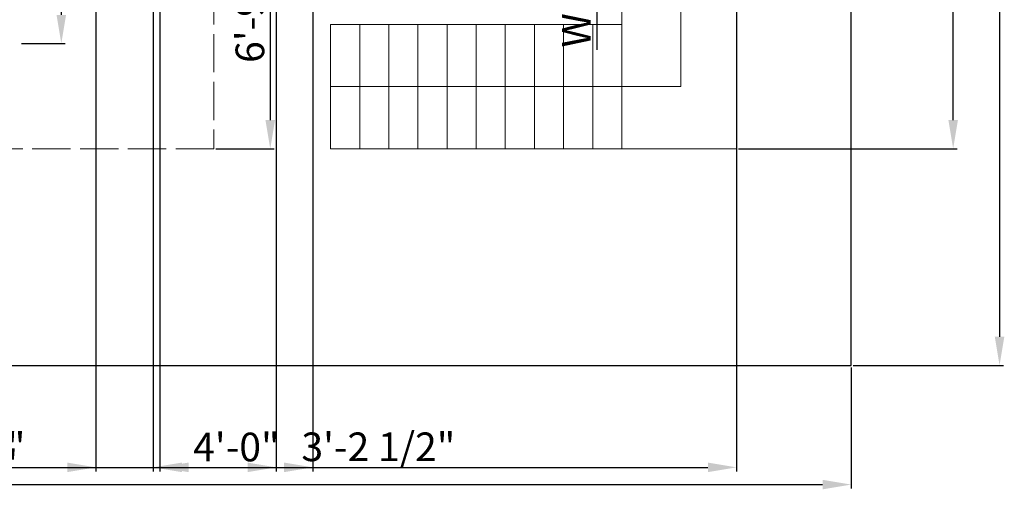
# Model space of a CAD drawing. Units: inches. Extents: x 2621 to 6190, y 513 to 1320.
# Tile 6 of 11: x 2997 to 3306, y 513 to 661. Entities that reach past the tile are written whole.
import ezdxf

# ---------------------------------------------------------------- set-up
doc = ezdxf.new("R2010")
doc.units = ezdxf.units.IN
doc.linetypes.add('ACAD_ISO02W100', pattern=[15, 12, -3])
for name, color, linetype, lineweight in [('A-ANNO-DIMS', 5, 'Continuous', 18), ('A-FLOR-PROJ', 1, 'ACAD_ISO02W100', 18), ('C-PROP', 7, 'Continuous', 25), ('stairs', 104, 'Continuous', 18)]:
    doc.layers.add(name, color=color, linetype=linetype, lineweight=lineweight)
doc.styles.get("Standard").update_dxf_attribs({"font": 'arial.ttf'})
doc.dimstyles.new('ISO-25', dxfattribs={"dimtxt": 9, "dimasz": 9, "dimexe": 1.25, "dimexo": 0.625, "dimtad": 1, "dimlunit": 3, "dimtxsty": 'Standard', "dimcen": 2.5, "dimadec": 0, "dimazin": 0, "dimtfac": 1, "dimtmove": 0, "dimatfit": 3, "dimfxl": 1, "dimarcsym": 0})

# ---------------------------------------------------------------- blocks, each defined once
blk = doc.blocks.new('*D33')
at = {"layer": 'A-ANNO-DIMS', "color": 0, "lineweight": -2, "transparency": 16777216}
for p, q in [((2997.94, 701.89), (3011.69, 701.89)), ((3010.44, 692.89), (3010.44, 662.89)), ((2997.94, 653.89), (3011.69, 653.89))]:
    blk.add_line(p, q, dxfattribs=at)
at = {"layer": 'A-ANNO-DIMS', "color": 0, "transparency": 16777216}
for points in [[(3008.94, 692.89), (3011.94, 692.89), (3010.44, 701.89)], [(3008.94, 662.89), (3011.94, 662.89), (3010.44, 653.89)]]:
    blk.add_solid(points, dxfattribs=at)
at = {"layer": 'Defpoints', "color": 0, "transparency": 16777216}
for p in [(2997.32, 701.89), (2997.32, 653.89), (3010.44, 653.89)]:
    blk.add_point(p, dxfattribs=at)
at = {"layer": 'A-ANNO-DIMS', "color": 0, "transparency": 16777216, "insert": (3005.32, 677.89), "char_height": 9, "attachment_point": 5, "rotation": 90}
blk.add_mtext("4'", dxfattribs=at)
blk = doc.blocks.new('*D34')
at = {"layer": 'A-ANNO-DIMS', "color": 0, "lineweight": -2, "transparency": 16777216}
for p, q in [((3058.97, 701.89), (3077.28, 701.89)), ((3076.03, 692.89), (3076.03, 629.89)), ((3058.97, 620.89), (3077.28, 620.89))]:
    blk.add_line(p, q, dxfattribs=at)
at = {"layer": 'A-ANNO-DIMS', "color": 0, "transparency": 16777216}
for points in [[(3074.53, 692.89), (3077.53, 692.89), (3076.03, 701.89)], [(3074.53, 629.89), (3077.53, 629.89), (3076.03, 620.89)]]:
    blk.add_solid(points, dxfattribs=at)
at = {"layer": 'Defpoints', "color": 0, "transparency": 16777216}
for p in [(3058.34, 701.89), (3058.34, 620.89), (3076.03, 620.89)]:
    blk.add_point(p, dxfattribs=at)
at = {"layer": 'A-ANNO-DIMS', "color": 0, "transparency": 16777216, "insert": (3070.81, 661.39), "char_height": 9, "attachment_point": 5, "rotation": 90}
blk.add_mtext('6\'-9"', dxfattribs=at)
blk = doc.blocks.new('*D37')
at = {"layer": 'A-ANNO-DIMS', "color": 0, "lineweight": -2, "transparency": 16777216}
for p, q in [((2718.38, 552.26), (2718.38, 514.23)), ((3258.38, 552.26), (3258.38, 514.23)), ((2727.38, 515.48), (3249.38, 515.48))]:
    blk.add_line(p, q, dxfattribs=at)
at = {"layer": 'A-ANNO-DIMS', "color": 0, "transparency": 16777216}
for points in [[(2727.38, 516.98), (2727.38, 513.98), (2718.38, 515.48)], [(3249.38, 516.98), (3249.38, 513.98), (3258.38, 515.48)]]:
    blk.add_solid(points, dxfattribs=at)
at = {"layer": 'Defpoints', "color": 0, "transparency": 16777216}
for p in [(2718.38, 552.89), (3258.38, 552.89), (3258.38, 515.48)]:
    blk.add_point(p, dxfattribs=at)
at = {"layer": 'A-ANNO-DIMS', "color": 0, "transparency": 16777216, "insert": (2988.38, 520.68), "char_height": 9, "attachment_point": 5}
blk.add_mtext("45'", dxfattribs=at)
blk = doc.blocks.new('*D39')
at = {"layer": 'A-ANNO-DIMS', "color": 0, "lineweight": -2, "transparency": 16777216}
for p, q in [((3259.01, 1121.89), (3306.19, 1121.89)), ((3304.94, 1112.89), (3304.94, 561.89)), ((3259.01, 552.89), (3306.19, 552.89))]:
    blk.add_line(p, q, dxfattribs=at)
at = {"layer": 'A-ANNO-DIMS', "color": 0, "transparency": 16777216}
for points in [[(3303.44, 1112.89), (3306.44, 1112.89), (3304.94, 1121.89)], [(3303.44, 561.89), (3306.44, 561.89), (3304.94, 552.89)]]:
    blk.add_solid(points, dxfattribs=at)
at = {"layer": 'Defpoints', "color": 0, "transparency": 16777216}
for p in [(3258.38, 1121.89), (3258.38, 552.89), (3304.94, 552.89)]:
    blk.add_point(p, dxfattribs=at)
at = {"layer": 'A-ANNO-DIMS', "color": 0, "transparency": 16777216, "insert": (3299.73, 837.39), "char_height": 9, "attachment_point": 5, "rotation": 90}
blk.add_mtext('47\'-5"', dxfattribs=at)
blk = doc.blocks.new('*D71')
at = {"layer": 'A-ANNO-DIMS', "color": 0, "lineweight": -2, "transparency": 16777216}
for p, q in [((3182.86, 743.94), (3177.28, 743.94)), ((3178.53, 734.94), (3178.53, 719.89)), ((3182.86, 710.89), (3177.28, 710.89)), ((3178.53, 710.89), (3178.53, 651.91))]:
    blk.add_line(p, q, dxfattribs=at)
at = {"layer": 'A-ANNO-DIMS', "color": 0, "transparency": 16777216}
for points in [[(3177.03, 734.94), (3180.03, 734.94), (3178.53, 743.94)], [(3177.03, 719.89), (3180.03, 719.89), (3178.53, 710.89)]]:
    blk.add_solid(points, dxfattribs=at)
at = {"layer": 'Defpoints', "color": 0, "transparency": 16777216}
for p in [(3183.49, 743.94), (3178.53, 710.89), (3183.49, 710.89)]:
    blk.add_point(p, dxfattribs=at)
at = {"layer": 'A-ANNO-DIMS', "color": 0, "transparency": 16777216, "insert": (3173.25, 676.9), "char_height": 9, "attachment_point": 5, "rotation": 90}
blk.add_mtext('WC 2\'-9"', dxfattribs=at)
blk = doc.blocks.new('*D86')
at = {"layer": 'A-ANNO-DIMS', "color": 0, "lineweight": -2, "transparency": 16777216}
for p, q in [((2898.87, 701.26), (2898.87, 519.64)), ((3021.32, 701.26), (3021.32, 519.64)), ((2907.87, 520.89), (3012.32, 520.89))]:
    blk.add_line(p, q, dxfattribs=at)
at = {"layer": 'A-ANNO-DIMS', "color": 0, "transparency": 16777216}
for points in [[(2907.87, 522.39), (2907.87, 519.39), (2898.87, 520.89)], [(3012.32, 522.39), (3012.32, 519.39), (3021.32, 520.89)]]:
    blk.add_solid(points, dxfattribs=at)
at = {"layer": 'Defpoints', "color": 0, "transparency": 16777216}
for p in [(2898.87, 701.89), (3021.32, 701.89), (3021.32, 520.89)]:
    blk.add_point(p, dxfattribs=at)
at = {"layer": 'A-ANNO-DIMS', "color": 0, "transparency": 16777216, "insert": (2960.09, 526.17), "char_height": 9, "attachment_point": 5}
blk.add_mtext('10\'-2 1/2"', dxfattribs=at)
blk = doc.blocks.new('*D91')
at = {"layer": 'A-ANNO-DIMS', "color": 0, "lineweight": -2, "transparency": 16777216}
for p, q in [((3223.01, 1085.89), (3291.63, 1085.89)), ((3290.38, 629.89), (3290.38, 1076.89)), ((3223.01, 620.89), (3291.63, 620.89))]:
    blk.add_line(p, q, dxfattribs=at)
at = {"layer": 'A-ANNO-DIMS', "color": 0, "transparency": 16777216}
for points in [[(3288.88, 1076.89), (3291.88, 1076.89), (3290.38, 1085.89)], [(3288.88, 629.89), (3291.88, 629.89), (3290.38, 620.89)]]:
    blk.add_solid(points, dxfattribs=at)
at = {"layer": 'Defpoints', "color": 0, "transparency": 16777216}
for p in [(3222.38, 1085.89), (3290.38, 1085.89), (3222.38, 620.89)]:
    blk.add_point(p, dxfattribs=at)
at = {"layer": 'A-ANNO-DIMS', "color": 0, "transparency": 16777216, "insert": (3285.16, 853.39), "char_height": 9, "attachment_point": 5, "rotation": 90}
blk.add_mtext('38\'-9"', dxfattribs=at)
blk = doc.blocks.new('*D92')
at = {"layer": 'A-ANNO-DIMS', "color": 0, "lineweight": -2, "transparency": 16777216}
for p, q in [((3222.38, 701.26), (3222.38, 519.64)), ((2730.38, 686.26), (2730.38, 519.64)), ((2739.38, 520.89), (3213.38, 520.89))]:
    blk.add_line(p, q, dxfattribs=at)
at = {"layer": 'A-ANNO-DIMS', "color": 0, "transparency": 16777216}
for points in [[(2739.38, 522.39), (2739.38, 519.39), (2730.38, 520.89)], [(3213.38, 522.39), (3213.38, 519.39), (3222.38, 520.89)]]:
    blk.add_solid(points, dxfattribs=at)
at = {"layer": 'Defpoints', "color": 0, "transparency": 16777216}
for p in [(3222.38, 701.89), (2730.38, 686.89), (3222.38, 520.89)]:
    blk.add_point(p, dxfattribs=at)
at = {"layer": 'A-ANNO-DIMS', "color": 0, "transparency": 16777216, "insert": (2976.38, 526.11), "char_height": 9, "attachment_point": 5}
blk.add_mtext('41\'-0"', dxfattribs=at)
blk = doc.blocks.new('*D102')
at = {"layer": 'A-ANNO-DIMS', "color": 0, "lineweight": -2, "transparency": 16777216}
for p, q in [((2915.57, 1054.4), (2915.57, 519.64)), ((2942.88, 1054.4), (2942.88, 519.64)), ((2924.57, 520.89), (2933.88, 520.89)), ((2942.88, 520.89), (2998.18, 520.89))]:
    blk.add_line(p, q, dxfattribs=at)
at = {"layer": 'A-ANNO-DIMS', "color": 0, "transparency": 16777216}
for points in [[(2924.57, 522.39), (2924.57, 519.39), (2915.57, 520.89)], [(2933.88, 522.39), (2933.88, 519.39), (2942.88, 520.89)]]:
    blk.add_solid(points, dxfattribs=at)
at = {"layer": 'Defpoints', "color": 0, "transparency": 16777216}
for p in [(2915.57, 1055.03), (2942.88, 1055.03), (2942.88, 520.89)]:
    blk.add_point(p, dxfattribs=at)
at = {"layer": 'A-ANNO-DIMS', "color": 0, "transparency": 16777216, "insert": (2975.03, 526.17), "char_height": 9, "attachment_point": 5}
blk.add_mtext('2\'-3 1/2"', dxfattribs=at)
blk = doc.blocks.new('*D107')
at = {"layer": 'A-ANNO-DIMS', "color": 0, "lineweight": -2, "transparency": 16777216}
for p, q in [((3041.38, 1076.26), (3041.38, 519.64)), ((3089.38, 1076.26), (3089.38, 519.64)), ((3050.38, 520.89), (3080.38, 520.89))]:
    blk.add_line(p, q, dxfattribs=at)
at = {"layer": 'A-ANNO-DIMS', "color": 0, "transparency": 16777216}
for points in [[(3050.38, 522.39), (3050.38, 519.39), (3041.38, 520.89)], [(3080.38, 522.39), (3080.38, 519.39), (3089.38, 520.89)]]:
    blk.add_solid(points, dxfattribs=at)
at = {"layer": 'Defpoints', "color": 0, "transparency": 16777216}
for p in [(3041.38, 1076.89), (3089.38, 1076.89), (3089.38, 520.89)]:
    blk.add_point(p, dxfattribs=at)
at = {"layer": 'A-ANNO-DIMS', "color": 0, "transparency": 16777216, "insert": (3065.38, 526.11), "char_height": 9, "attachment_point": 5}
blk.add_mtext('4\'-0"', dxfattribs=at)
blk = doc.blocks.new('*D108')
at = {"layer": 'A-ANNO-DIMS', "color": 0, "lineweight": -2, "transparency": 16777216}
for p, q in [((3039.32, 701.26), (3039.32, 519.64)), ((3077.89, 701.26), (3077.89, 519.64)), ((3048.32, 520.89), (3068.89, 520.89)), ((3077.89, 520.89), (3133.03, 520.89))]:
    blk.add_line(p, q, dxfattribs=at)
at = {"layer": 'A-ANNO-DIMS', "color": 0, "transparency": 16777216}
for points in [[(3048.32, 522.39), (3048.32, 519.39), (3039.32, 520.89)], [(3068.89, 522.39), (3068.89, 519.39), (3077.89, 520.89)]]:
    blk.add_solid(points, dxfattribs=at)
at = {"layer": 'Defpoints', "color": 0, "transparency": 16777216}
for p in [(3039.32, 701.89), (3077.89, 701.89), (3077.89, 520.89)]:
    blk.add_point(p, dxfattribs=at)
at = {"layer": 'A-ANNO-DIMS', "color": 0, "transparency": 16777216, "insert": (3109.96, 526.17), "char_height": 9, "attachment_point": 5}
blk.add_mtext('3\'-2 1/2"', dxfattribs=at)

msp = doc.modelspace()

# ---------------------------------------------------------------- linework, layer by layer
at = {"layer": 'A-FLOR-PROJ'}
msp.add_lwpolyline([(3058.344, 701.89), (3058.344, 620.89), (2730.381, 620.89), (2730.381, 782.89)], dxfattribs=at)
at = {"layer": 'C-PROP'}
msp.add_lwpolyline([(3258.381, 552.89), (3258.381, 1121.89), (2742.381, 1121.89), (2718.381, 552.89)], close=True, dxfattribs=at)
at = {"layer": 'stairs'}
for p, q in [((3186.381, 701.89), (3186.381, 620.89)), ((3222.381, 701.89), (3222.381, 620.89)), ((3204.871, 640.39), (3204.871, 682.39)), ((3094.96, 659.89), (3094.96, 620.89)), ((3186.381, 659.89), (3094.96, 659.89)), ((3104.102, 659.89), (3104.102, 620.89)), ((3113.244, 659.89), (3113.244, 620.89)), ((3122.386, 659.89), (3122.386, 620.89)), ((3131.528, 659.89), (3131.528, 620.89)), ((3140.67, 659.89), (3140.67, 620.89)), ((3149.813, 659.89), (3149.813, 620.89)), ((3158.955, 659.89), (3158.955, 620.89)), ((3168.097, 659.89), (3168.097, 620.89)), ((3177.239, 659.89), (3177.239, 620.89)), ((3186.381, 659.89), (3186.381, 620.89)), ((3094.96, 640.39), (3204.871, 640.39)), ((3094.96, 620.89), (3108.983, 620.89)), ((3222.381, 620.89), (3108.983, 620.89))]:
    msp.add_line(p, q, dxfattribs=at)

# ---------------------------------------------------------------- dimensions: what is measured, and where the dimension line sits
at = {"layer": 'A-ANNO-DIMS'}
for base, p1, p2, override, picture, middle in [((3304.936, 552.89), (3258.381, 1121.89), (3258.381, 552.89), {"dimclrd": 0, "dimclre": 0, "dimclrt": 0}, '*D39', (3299.735, 837.39)), ((3290.381, 1085.89), (3222.381, 620.89), (3222.381, 1085.89), {"dimdec": 1, "dimlfac": 1, "dimrnd": 0, "dimzin": 1, "dimdsep": 46, "dimlunit": 4, "dimfrac": 2}, '*D91', (3285.158, 853.39)), ((3010.445, 653.89), (2997.318, 701.89), (2997.318, 653.89), {"dimclrd": 0, "dimclre": 0, "dimclrt": 0}, '*D33', (3005.32, 677.89)), ((3076.033, 620.89), (3058.344, 701.89), (3058.344, 620.89), {"dimclrd": 0, "dimclre": 0, "dimclrt": 0}, '*D34', (3070.812, 661.39))]:
    dim = msp.add_linear_dim(base=base, p1=p1, p2=p2, angle=90, dimstyle='ISO-25', override=override, dxfattribs=at)
    dim.commit()
    dim.dimension.update_dxf_attribs({"geometry": picture, "text_midpoint": middle})
for base, p1, p2, override, picture, middle in [((3089.381, 520.89), (3041.381, 1076.89), (3089.381, 1076.89), {"dimdec": 1, "dimlfac": 1, "dimrnd": 0, "dimzin": 1, "dimdsep": 46, "dimlunit": 4, "dimfrac": 2}, '*D107', (3065.381, 526.11)), ((2942.877, 520.89), (2915.573, 1055.025), (2942.877, 1055.025), {"dimdec": 1, "dimlfac": 1, "dimrnd": 0, "dimzin": 1, "dimdsep": 46, "dimlunit": 4, "dimfrac": 2}, '*D102', (2975.027, 526.171)), ((3222.381, 520.89), (2730.381, 686.89), (3222.381, 701.89), {"dimdec": 1, "dimlfac": 1, "dimrnd": 0, "dimzin": 1, "dimdsep": 46, "dimlunit": 4, "dimfrac": 2}, '*D92', (2976.381, 526.11)), ((3021.318, 520.89), (2898.869, 701.89), (3021.318, 701.89), {"dimdec": 1, "dimlfac": 1, "dimrnd": 0, "dimzin": 1, "dimdsep": 46, "dimlunit": 4, "dimfrac": 2}, '*D86', (2960.094, 526.168)), ((3077.887, 520.89), (3039.318, 701.89), (3077.887, 701.89), {"dimdec": 1, "dimlfac": 1, "dimrnd": 0, "dimzin": 1, "dimdsep": 46, "dimlunit": 4, "dimfrac": 2}, '*D108', (3109.957, 526.171)), ((3258.381, 515.475), (2718.381, 552.89), (3258.381, 552.89), {"dimclrd": 0, "dimclre": 0, "dimclrt": 0}, '*D37', (2988.381, 520.677))]:
    dim = msp.add_linear_dim(base=base, p1=p1, p2=p2, dimstyle='ISO-25', override=override, dxfattribs=at)
    dim.commit()
    dim.dimension.update_dxf_attribs({"geometry": picture, "text_midpoint": middle})
dim = msp.add_linear_dim(base=(3178.531, 710.89), p1=(3183.488, 743.936), p2=(3183.488, 710.89), angle=270, text='WC <>', dimstyle='ISO-25', override={"dimdec": 1, "dimlfac": 1, "dimrnd": 0, "dimzin": 1, "dimdsep": 46, "dimlunit": 4, "dimfrac": 2}, dxfattribs=at)
dim.commit()
dim.dimension.update_dxf_attribs({"geometry": '*D71', "text_midpoint": (3173.253, 676.898)})

doc.saveas('drawing.dxf')
